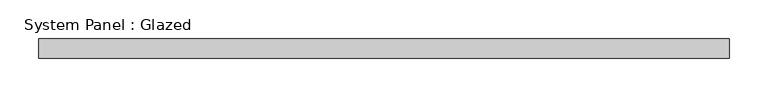
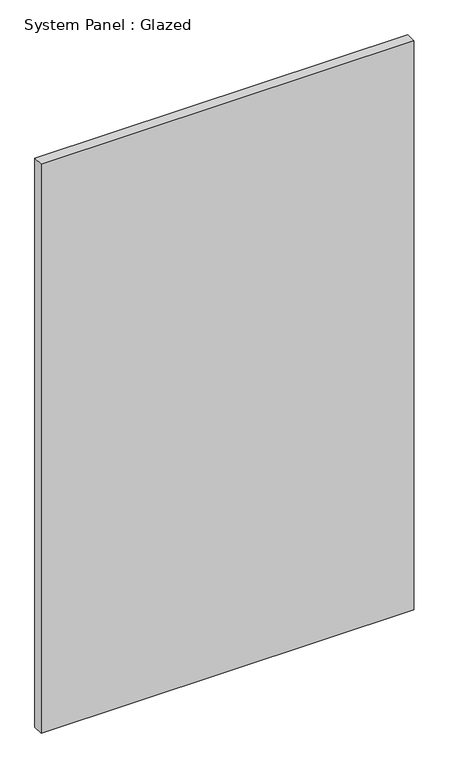
"""IFC4 building model written with IfcOpenShell, lengths in millimetres: plate geometry, System Panel : Glazed."""

from ifc_helpers import new_model, si_unit, origin, origin_with_axes, place, context, project, spatial, polyline, outline, extrude, source, transform, mapped, element, save


def system_panel_glazed_27a553ef(model_context):
    return source(origin(), model_context, "Body", "SweptSolid", [
        extrude(outline(polyline([(447.675, 19.05), (-447.675, 19.05), (-447.675, 44.45), (447.675, 44.45), (447.675, 19.05)])), origin_with_axes(), (0.0, 0.0, 1.0), 1443.4687519),
    ])


if __name__ == "__main__":
    model = new_model("IFC4")
    model_context = context("Model", 3, world=origin())
    ifc_project = project(units=[si_unit("LENGTHUNIT", "METRE", prefix="MILLI")], contexts=[model_context])
    site = spatial("IfcSite", under=ifc_project)
    building = spatial("IfcBuilding", under=site)
    placement = place(None, origin())
    system_panel_glazed_shape = system_panel_glazed_27a553ef(model_context)
    element("IfcPlate", 1, ObjectType="System Panel : Glazed", at=placement, inside=building, context=model_context, shape_type="MappedRepresentation", body=[
        mapped(system_panel_glazed_shape, transform((0.0, 0.0, 0.0), x_axis=(1.0, 0.0, 0.0), y_axis=(0.0, 1.0, 0.0), z_axis=(0.0, 0.0, 1.0))),
    ])
    save(model, "model.ifc")

# Revit data of these elements
# Type "System Panel : Glazed"
#   Construction Type Id = "GSP4R"
#   Analytic Construction = "1/8 in Pilkington single glazing"
#   Visual Light Transmittance = 0.9
#   Solar Heat Gain Coefficient = 0.86
#   Heat Transfer Coefficient (U) = 1.18115 BTU/(h·ft²·°F)
#   Define Thermal Properties by = 1
# Element 1 (IfcPlate, "System Panel : Glazed")
#   Materials on its faces: "Glass"
# Materials
#   "Glass": class "Glass", colour RGB 0 128 192, transparency 0.75, Description = "Soda Lime Glass", Cost = 0
